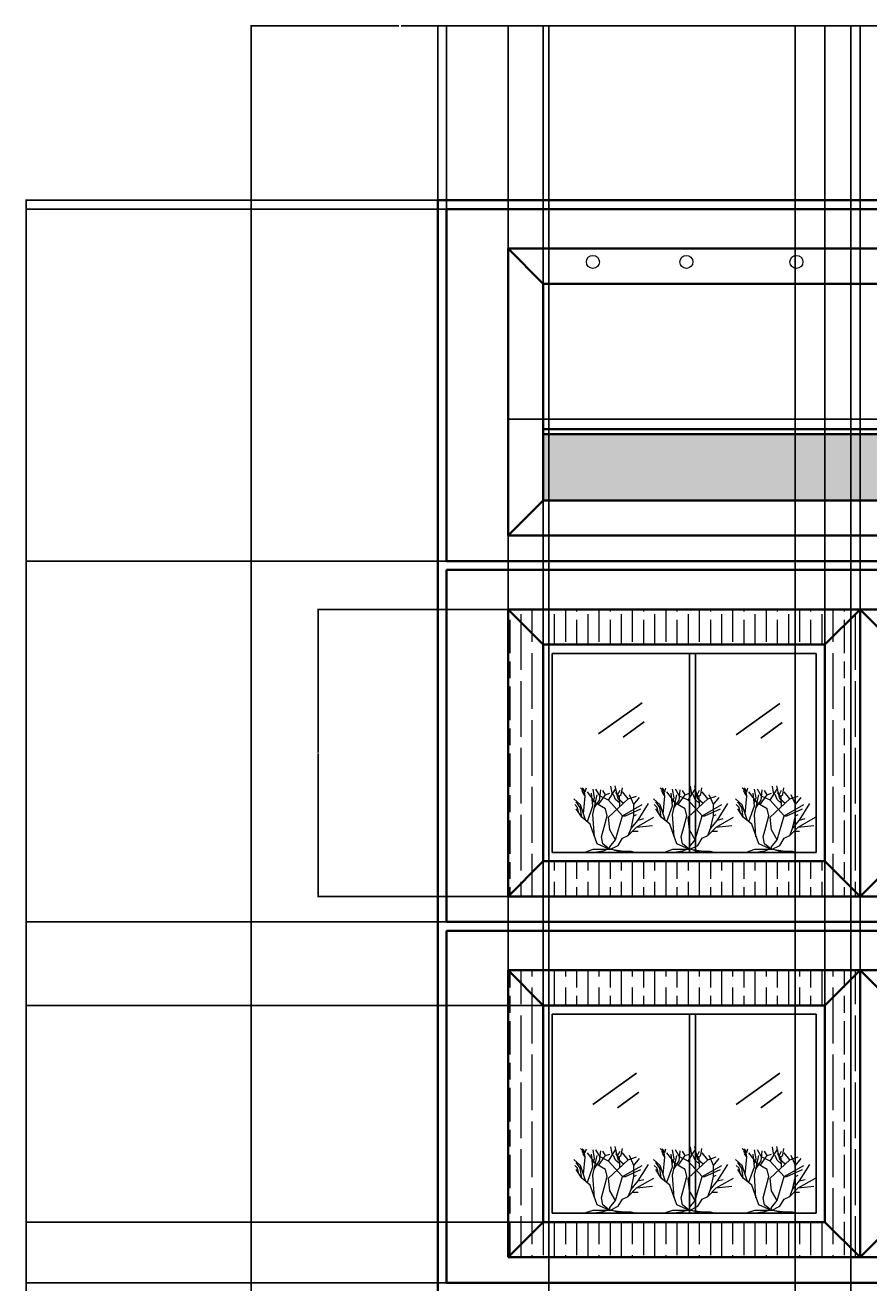
# Model space of a CAD drawing. Units: inches. Extents: x -97 to 1206, y -378 to 680.
# Tile 4 of 6: x -97 to 191, y 251 to 680. Entities that reach past the tile are written whole.
import ezdxf

# ---------------------------------------------------------------- set-up
doc = ezdxf.new("R2010")
doc.units = ezdxf.units.IN
doc.header["$MEASUREMENT"] = 0
for name, color, linetype, lineweight in [('A-ANNO-DIMS', 2, 'Continuous', 18), ('A-ELEV', 7, 'Continuous', 35), ('A-ELEV-PATT', 252, 'Continuous', 13), ('A-GLAZ', 4, 'Continuous', 25), ('E-LITE', 2, 'Continuous', 18), ('L-PLNT', 82, 'Continuous', 13)]:
    doc.layers.add(name, color=color, linetype=linetype, lineweight=lineweight)
doc.styles.get("Standard").update_dxf_attribs({"font": 'arial.ttf'})
doc.dimstyles.get("Standard").update_dxf_attribs({"dimtxt": 0.18, "dimasz": 0.18, "dimexe": 0.18, "dimexo": 0.0625, "dimgap": 0.09, "dimtad": 0, "dimtih": 1, "dimtoh": 1, "dimdec": 4, "dimzin": 0, "dimdsep": 46, "dimtxsty": 'Standard', "dimcen": 0.09, "dimadec": 0, "dimazin": 0, "dimtfac": 1, "dimtdec": 4, "dimtofl": 0, "dimtmove": 0, "dimatfit": 3, "dimfxl": 1, "dimtolj": 1, "dimtzin": 0, "dimarcsym": 0})

# ---------------------------------------------------------------- blocks, each defined once
blk = doc.blocks.new('*U2')
for p, q in [((-12.471, 19.775), (-12.898, 22.044)), ((-11.433, 18.289), (-10.457, 22.749)), ((-8.16, 17.76), (-10.56, 21.6)), ((-9.48, 19.775), (-8.992, 22.592)), ((-5.28, 19.2), (-3.84, 21.6)), ((-3.377, 18.602), (-2.888, 21.575)), ((-0.508, 21.888), (-0.081, 20.558)), ((0.041, 20.714), (1.384, 22.044)), ((0.102, 21.34), (0.835, 21.888)), ((-16.8, 16.32), (-18.72, 18.72)), ((-14.88, 18.24), (-17.76, 19.2)), ((-16.8, 16.32), (-15.36, 19.68)), ((-14.88, 18.24), (-12.96, 20.64)), ((-8.16, 12), (-14.88, 18.24)), ((-13.325, 16.724), (-11.433, 18.289)), ((-12.96, 12.48), (-8.16, 17.76)), ((-11.677, 19.071), (-12.471, 19.775)), ((-11.28, 19.619), (-12.104, 21.184)), ((-12.043, 15.628), (-11.921, 18.836)), ((-11.982, 16.802), (-10.579, 18.054)), ((-11.921, 18.836), (-10.64, 20.401)), ((-10.579, 18.054), (-9.846, 19.697)), ((-7.2, 19.68), (-8.64, 20.16)), ((-8.16, 17.76), (-5.28, 19.2)), ((-7.2, 19.68), (-6.24, 21.12)), ((-4.8, 16.32), (-7.2, 19.68)), ((-5.086, 17.741), (-5.513, 21.34)), ((-3.377, 15.315), (-5.086, 17.819)), ((-2.88, 12.96), (-4.32, 19.68)), ((-3.84, 16.8), (-0.96, 20.64)), ((-2.766, 16.802), (-3.377, 18.602)), ((-2.88, 15.84), (-2.4, 20.16)), ((-0.203, 19.149), (0.102, 21.34)), ((0.346, 13.203), (-0.203, 19.149)), ((-0.142, 19.384), (0.59, 20.401)), ((-0.02, 20.01), (0.896, 21.105)), ((1.323, 16.254), (3.642, 18.289)), ((1.44, 15.36), (2.88, 17.28)), ((-18.24, 11.04), (-21.755, 16.655)), ((-12.96, 12.48), (-19.68, 16.32)), ((-13.92, 12.48), (-19.2, 14.88)), ((-16.8, 12.48), (-17.76, 12.96)), ((-16.8, 12.48), (-16.8, 16.32)), ((-7.68, 12.48), (-7.2, 14.88)), ((-7.2, 14.88), (-3.84, 16.8)), ((-3.36, 5.28), (-2.88, 12.96)), ((-0.96, 10.56), (-2.88, 15.84)), ((-0.48, 10.8), (0.346, 13.203)), ((0.346, 13.203), (1.323, 16.254)), ((0.96, 12), (1.44, 15.36)), ((0.96, 12), (2.88, 14.88)), ((1.92, 13.44), (2.4, 15.36)), ((2.4, 15.36), (3.36, 16.32)), ((-17.76, 8.64), (-23.663, 11.961)), ((-17.76, 8.64), (-23.128, 9.222)), ((-18.24, 11.04), (-20.16, 11.52)), ((-15.84, 8.16), (-18.24, 11.04)), ((-14.88, 5.76), (-17.76, 8.64)), ((-15.84, 8.16), (-16.8, 12.48)), ((-12.96, 12.48), (-13.92, 12.48)), ((-10.56, 4.32), (-12.96, 12.48)), ((-8.64, 7.68), (-8.16, 12)), ((-6.72, 8.64), (-7.68, 12.48)), ((-5.76, 5.28), (-6.72, 8.64)), ((-4.32, 2.88), (-1.92, 9.6)), ((-1.92, 9.6), (0.96, 12)), ((-16.32, 7.2), (-18.24, 7.2)), ((-14.88, 5.76), (-15.84, 8.16)), ((-12.96, 4.8), (-14.88, 5.76)), ((-11.52, 2.4), (-12.96, 4.8)), ((-10.56, 4.32), (-8.64, 7.68)), ((-8.64, 1.92), (-10.56, 4.32)), ((-6.24, 2.88), (-5.76, 5.28)), ((-15.84, 0.48), (-17.76, 0)), ((-13.44, 0.48), (-15.84, 0.48)), ((-9.6, 0.96), (-13.44, 0.48)), ((-9.6, 0.96), (-12.96, 0)), ((-8.64, 0.96), (-11.52, 2.4)), ((-9.6, 0.96), (-7.68, 0.96)), ((-8.64, 0.96), (-4.32, 2.88)), ((-8.64, 0.96), (-6.24, 2.88)), ((-8.64, 0.96), (-8.64, 1.92)), ((-8.64, 0.96), (-2.88, 0.96)), ((-7.68, 0.96), (-6.24, 0.48)), ((-6.24, 0.48), (-3.36, 0)), ((-2.88, 0.96), (0, 0))]:
    blk.add_line(p, q)
blk = doc.blocks.new('FACADE-SURROUND')
for p, q in [((432, 97.83), (0, 97.83)), ((0, 97.83), (0, 0)), ((12, 85.83), (0, 97.83)), ((300, 85.83), (312, 97.83)), ((312, 0), (312, 97.83)), ((312, 0), (312, 97.83)), ((312, 97.83), (324, 85.83)), ((432, 97.83), (420, 85.83)), ((432, 0), (432, 97.83)), ((12, 85.83), (12, 12)), ((108, 85.83), (12, 85.83)), ((300, 85.83), (126, 85.83)), ((126, 85.83), (126, 12)), ((300, 12), (300, 85.83)), ((324, 12), (324, 85.83)), ((420, 85.83), (324, 85.83)), ((420, 12), (420, 85.83)), ((12, 12), (0, 0)), ((12, 12), (108, 12)), ((126, 12), (300, 12)), ((300, 12), (312, 0)), ((312, 0), (324, 12)), ((324, 12), (420, 12)), ((432, 0), (420, 12)), ((0, 0), (432, 0))]:
    blk.add_line(p, q)
blk = doc.blocks.new('WIN-1500')
for p, q in [((90, 67.83), (0, 67.83)), ((0, 67.83), (0, 0)), ((90, 67.83), (90, 0)), ((0, 0), (90, 0))]:
    blk.add_line(p, q)
blk = doc.blocks.new('*D9')
at = {"layer": 'A-ANNO-DIMS', "color": 0, "lineweight": -2, "transparency": 16777216}
for p, q in [((67.93, 480.46), (67.93, 545.38)), ((68.11, 545.2), (282.03, 545.2)), ((499.75, 545.2), (285.83, 545.2)), ((499.93, 480.46), (499.93, 545.38))]:
    blk.add_line(p, q, dxfattribs=at)
at = {"layer": 'A-ANNO-DIMS', "color": 0, "transparency": 16777216}
for points in [[(68.11, 545.23), (68.11, 545.17), (67.93, 545.2)], [(499.75, 545.23), (499.75, 545.17), (499.93, 545.2)]]:
    blk.add_solid(points, dxfattribs=at)
at = {"layer": 'Defpoints', "color": 0, "transparency": 16777216}
for p in [(67.93, 545.2), (67.93, 480.4), (499.93, 480.4)]:
    blk.add_point(p, dxfattribs=at)
at = {"layer": 'A-ANNO-DIMS', "color": 0, "transparency": 16777216, "insert": (283.93, 545.2), "char_height": 0.18, "attachment_point": 5}
blk.add_mtext('\\A1;FACADE SURROUND 432 TYP.', dxfattribs=at)
blk = doc.blocks.new('*D10')
at = {"layer": 'A-ANNO-DIMS', "color": 0, "lineweight": -2, "transparency": 16777216}
for p, q in [((67.86, 480.4), (2.95, 480.4)), ((3.13, 480.22), (3.13, 431.66)), ((3.13, 382.75), (3.13, 431.3)), ((67.86, 382.57), (2.95, 382.57))]:
    blk.add_line(p, q, dxfattribs=at)
at = {"layer": 'A-ANNO-DIMS', "color": 0, "transparency": 16777216}
for points in [[(3.1, 480.22), (3.16, 480.22), (3.13, 480.4)], [(3.1, 382.75), (3.16, 382.75), (3.13, 382.57)]]:
    blk.add_solid(points, dxfattribs=at)
at = {"layer": 'Defpoints', "color": 0, "transparency": 16777216}
for p in [(67.93, 480.4), (3.13, 382.57), (67.93, 382.57)]:
    blk.add_point(p, dxfattribs=at)
at = {"layer": 'A-ANNO-DIMS', "color": 0, "transparency": 16777216, "insert": (3.13, 431.48), "char_height": 0.18, "attachment_point": 5}
blk.add_mtext('\\A1;98 TYP.', dxfattribs=at)
blk = doc.blocks.new('*D12')
at = {"layer": 'A-ANNO-DIMS', "color": 0, "lineweight": -2, "transparency": 16777216}
for p, q in [((43.86, 619.86), (-96.59, 619.86)), ((-96.41, 619.68), (-96.41, 252.54)), ((-96.41, -114.96), (-96.41, 252.17)), ((-36.97, -115.14), (-96.59, -115.14))]:
    blk.add_line(p, q, dxfattribs=at)
at = {"layer": 'A-ANNO-DIMS', "color": 0, "transparency": 16777216}
for points in [[(-96.44, 619.68), (-96.38, 619.68), (-96.41, 619.86)], [(-96.44, -114.96), (-96.38, -114.96), (-96.41, -115.14)]]:
    blk.add_solid(points, dxfattribs=at)
at = {"layer": 'Defpoints', "color": 0, "transparency": 16777216}
for p in [(43.93, 619.86), (-96.41, -115.14), (-36.91, -115.14)]:
    blk.add_point(p, dxfattribs=at)
at = {"layer": 'A-ANNO-DIMS', "color": 0, "transparency": 16777216, "insert": (-96.41, 252.36), "char_height": 0.18, "attachment_point": 5}
blk.add_mtext('\\A1;735', dxfattribs=at)
blk = doc.blocks.new('*D16')
at = {"layer": 'A-ANNO-DIMS', "color": 0, "lineweight": -2, "transparency": 16777216}
for p, q in [((46.86, 373.86), (-96.59, 373.86)), ((-96.41, 373.68), (-96.41, 312.54)), ((-96.41, 251.04), (-96.41, 312.17)), ((46.86, 250.86), (-96.59, 250.86))]:
    blk.add_line(p, q, dxfattribs=at)
at = {"layer": 'A-ANNO-DIMS', "color": 0, "transparency": 16777216}
for points in [[(-96.44, 373.68), (-96.38, 373.68), (-96.41, 373.86)], [(-96.44, 251.04), (-96.38, 251.04), (-96.41, 250.86)]]:
    blk.add_solid(points, dxfattribs=at)
at = {"layer": 'Defpoints', "color": 0, "transparency": 16777216}
for p in [(-96.41, 373.86), (46.93, 373.86), (46.93, 250.86)]:
    blk.add_point(p, dxfattribs=at)
at = {"layer": 'A-ANNO-DIMS', "color": 0, "transparency": 16777216, "insert": (-96.41, 312.36), "char_height": 0.18, "attachment_point": 5}
blk.add_mtext('\\A1;123', dxfattribs=at)
blk = doc.blocks.new('*D17')
at = {"layer": 'A-ANNO-DIMS', "color": 0, "lineweight": -2, "transparency": 16777216}
for p, q in [((46.86, 496.86), (-96.59, 496.86)), ((-96.41, 496.68), (-96.41, 435.54)), ((-96.41, 374.04), (-96.41, 435.17)), ((46.86, 373.86), (-96.59, 373.86))]:
    blk.add_line(p, q, dxfattribs=at)
at = {"layer": 'A-ANNO-DIMS', "color": 0, "transparency": 16777216}
for points in [[(-96.44, 496.68), (-96.38, 496.68), (-96.41, 496.86)], [(-96.44, 374.04), (-96.38, 374.04), (-96.41, 373.86)]]:
    blk.add_solid(points, dxfattribs=at)
at = {"layer": 'Defpoints', "color": 0, "transparency": 16777216}
for p in [(-96.41, 496.86), (46.93, 496.86), (46.93, 373.86)]:
    blk.add_point(p, dxfattribs=at)
at = {"layer": 'A-ANNO-DIMS', "color": 0, "transparency": 16777216, "insert": (-96.41, 435.36), "char_height": 0.18, "attachment_point": 5}
blk.add_mtext('\\A1;123', dxfattribs=at)
blk = doc.blocks.new('*D18')
at = {"layer": 'A-ANNO-DIMS', "color": 0, "lineweight": -2, "transparency": 16777216}
for p, q in [((46.86, 616.86), (-96.59, 616.86)), ((-96.41, 616.68), (-96.41, 557.04)), ((-96.41, 497.04), (-96.41, 556.67)), ((46.86, 496.86), (-96.59, 496.86))]:
    blk.add_line(p, q, dxfattribs=at)
at = {"layer": 'A-ANNO-DIMS', "color": 0, "transparency": 16777216}
for points in [[(-96.44, 616.68), (-96.38, 616.68), (-96.41, 616.86)], [(-96.44, 497.04), (-96.38, 497.04), (-96.41, 496.86)]]:
    blk.add_solid(points, dxfattribs=at)
at = {"layer": 'Defpoints', "color": 0, "transparency": 16777216}
for p in [(-96.41, 616.86), (46.93, 616.86), (46.93, 496.86)]:
    blk.add_point(p, dxfattribs=at)
at = {"layer": 'A-ANNO-DIMS', "color": 0, "transparency": 16777216, "insert": (-96.41, 556.86), "char_height": 0.18, "attachment_point": 5}
blk.add_mtext('\\A1;120', dxfattribs=at)
blk = doc.blocks.new('*D31')
at = {"layer": 'A-ANNO-DIMS', "color": 0, "lineweight": -2, "transparency": 16777216}
for p, q in [((46.93, 616.92), (46.93, 679.54)), ((47.11, 679.36), (57.22, 679.36)), ((67.75, 679.36), (57.63, 679.36)), ((67.93, 603.46), (67.93, 679.54))]:
    blk.add_line(p, q, dxfattribs=at)
at = {"layer": 'A-ANNO-DIMS', "color": 0, "transparency": 16777216}
for points in [[(47.11, 679.39), (47.11, 679.33), (46.93, 679.36)], [(67.75, 679.39), (67.75, 679.33), (67.93, 679.36)]]:
    blk.add_solid(points, dxfattribs=at)
at = {"layer": 'Defpoints', "color": 0, "transparency": 16777216}
for p in [(67.93, 679.36), (46.93, 616.86), (67.93, 603.4)]:
    blk.add_point(p, dxfattribs=at)
at = {"layer": 'A-ANNO-DIMS', "color": 0, "transparency": 16777216, "insert": (57.43, 679.36), "char_height": 0.18, "attachment_point": 5}
blk.add_mtext('\\A1;21', dxfattribs=at)
blk = doc.blocks.new('*D32')
at = {"layer": 'A-ANNO-DIMS', "color": 0, "lineweight": -2, "transparency": 16777216}
for p, q in [((67.93, 603.46), (67.93, 679.54)), ((68.11, 679.36), (229.64, 679.36)), ((391.75, 679.36), (230.21, 679.36)), ((391.93, 603.46), (391.93, 679.54))]:
    blk.add_line(p, q, dxfattribs=at)
at = {"layer": 'A-ANNO-DIMS', "color": 0, "transparency": 16777216}
for points in [[(68.11, 679.39), (68.11, 679.33), (67.93, 679.36)], [(391.75, 679.39), (391.75, 679.33), (391.93, 679.36)]]:
    blk.add_solid(points, dxfattribs=at)
at = {"layer": 'Defpoints', "color": 0, "transparency": 16777216}
for p in [(391.93, 679.36), (67.93, 603.4), (391.93, 603.4)]:
    blk.add_point(p, dxfattribs=at)
at = {"layer": 'A-ANNO-DIMS', "color": 0, "transparency": 16777216, "insert": (229.93, 679.36), "char_height": 0.18, "attachment_point": 5}
blk.add_mtext('\\A1;324', dxfattribs=at)
blk = doc.blocks.new('*D36')
at = {"layer": 'A-ANNO-DIMS', "color": 0, "lineweight": -2, "transparency": 16777216}
for p, q in [((-19.68, -48.26), (-19.68, 679.54)), ((-19.5, 679.36), (30.69, 679.36)), ((81.65, 679.36), (31.46, 679.36)), ((81.83, -48.26), (81.83, 679.54))]:
    blk.add_line(p, q, dxfattribs=at)
at = {"layer": 'A-ANNO-DIMS', "color": 0, "transparency": 16777216}
for points in [[(-19.5, 679.39), (-19.5, 679.33), (-19.68, 679.36)], [(81.65, 679.39), (81.65, 679.33), (81.83, 679.36)]]:
    blk.add_solid(points, dxfattribs=at)
at = {"layer": 'Defpoints', "color": 0, "transparency": 16777216}
for p in [(81.83, 679.36), (-19.68, -48.33), (81.83, -48.33)]:
    blk.add_point(p, dxfattribs=at)
at = {"layer": 'A-ANNO-DIMS', "color": 0, "transparency": 16777216, "insert": (31.08, 679.36), "char_height": 0.18, "attachment_point": 5}
blk.add_mtext('\\A1;101.5', dxfattribs=at)
blk = doc.blocks.new('*D45')
at = {"layer": 'A-ANNO-DIMS', "color": 0, "lineweight": -2, "transparency": 16777216}
for p, q in [((43.93, -24.66), (43.93, 679.54)), ((44.11, 679.36), (104.5, 679.36)), ((165.65, 679.36), (105.27, 679.36)), ((165.83, -24.66), (165.83, 679.54))]:
    blk.add_line(p, q, dxfattribs=at)
at = {"layer": 'A-ANNO-DIMS', "color": 0, "transparency": 16777216}
for points in [[(44.11, 679.39), (44.11, 679.33), (43.93, 679.36)], [(165.65, 679.39), (165.65, 679.33), (165.83, 679.36)]]:
    blk.add_solid(points, dxfattribs=at)
at = {"layer": 'Defpoints', "color": 0, "transparency": 16777216}
for p in [(165.83, 679.36), (43.93, -24.73), (165.83, -24.73)]:
    blk.add_point(p, dxfattribs=at)
at = {"layer": 'A-ANNO-DIMS', "color": 0, "transparency": 16777216, "insert": (104.88, 679.36), "char_height": 0.18, "attachment_point": 5}
blk.add_mtext('\\A1;121.9', dxfattribs=at)
blk = doc.blocks.new('*D46')
at = {"layer": 'A-ANNO-DIMS', "color": 0, "lineweight": -2, "transparency": 16777216}
for p, q in [((165.83, -24.66), (165.83, 679.54)), ((166.01, 679.36), (174.88, 679.36)), ((184.65, 679.36), (175.79, 679.36)), ((184.83, -24.66), (184.83, 679.54))]:
    blk.add_line(p, q, dxfattribs=at)
at = {"layer": 'A-ANNO-DIMS', "color": 0, "transparency": 16777216}
for points in [[(166.01, 679.39), (166.01, 679.33), (165.83, 679.36)], [(184.65, 679.39), (184.65, 679.33), (184.83, 679.36)]]:
    blk.add_solid(points, dxfattribs=at)
at = {"layer": 'Defpoints', "color": 0, "transparency": 16777216}
for p in [(184.83, 679.36), (165.83, -24.73), (184.83, -24.73)]:
    blk.add_point(p, dxfattribs=at)
at = {"layer": 'A-ANNO-DIMS', "color": 0, "transparency": 16777216, "insert": (175.33, 679.36), "char_height": 0.18, "attachment_point": 5}
blk.add_mtext('\\A1;18.994', dxfattribs=at)
blk = doc.blocks.new('*D47')
at = {"layer": 'A-ANNO-DIMS', "color": 0, "lineweight": -2, "transparency": 16777216}
for p, q in [((184.83, -24.66), (184.83, 679.54)), ((185.01, 679.36), (255.01, 679.36)), ((325.75, 679.36), (255.75, 679.36)), ((325.93, -24.66), (325.93, 679.54))]:
    blk.add_line(p, q, dxfattribs=at)
at = {"layer": 'A-ANNO-DIMS', "color": 0, "transparency": 16777216}
for points in [[(185.01, 679.39), (185.01, 679.33), (184.83, 679.36)], [(325.75, 679.39), (325.75, 679.33), (325.93, 679.36)]]:
    blk.add_solid(points, dxfattribs=at)
at = {"layer": 'Defpoints', "color": 0, "transparency": 16777216}
for p in [(325.93, 679.36), (184.83, -24.73), (325.93, -24.73)]:
    blk.add_point(p, dxfattribs=at)
at = {"layer": 'A-ANNO-DIMS', "color": 0, "transparency": 16777216, "insert": (255.38, 679.36), "char_height": 0.18, "attachment_point": 5}
blk.add_mtext('\\A1;141.1', dxfattribs=at)
blk = doc.blocks.new('*D51')
at = {"layer": 'A-ANNO-DIMS', "color": 0, "lineweight": -2, "transparency": 16777216}
for p, q in [((67.93, 357.46), (67.93, 679.54)), ((68.11, 679.36), (73.54, 679.36)), ((79.75, 679.36), (74.31, 679.36)), ((79.93, 345.46), (79.93, 679.54))]:
    blk.add_line(p, q, dxfattribs=at)
at = {"layer": 'A-ANNO-DIMS', "color": 0, "transparency": 16777216}
for points in [[(68.11, 679.39), (68.11, 679.33), (67.93, 679.36)], [(79.75, 679.39), (79.75, 679.33), (79.93, 679.36)]]:
    blk.add_solid(points, dxfattribs=at)
at = {"layer": 'Defpoints', "color": 0, "transparency": 16777216}
for p in [(79.93, 679.36), (67.93, 357.4), (79.93, 345.4)]:
    blk.add_point(p, dxfattribs=at)
at = {"layer": 'A-ANNO-DIMS', "color": 0, "transparency": 16777216, "insert": (73.93, 679.36), "char_height": 0.18, "attachment_point": 5}
blk.add_mtext('\\A1;12.00', dxfattribs=at)
blk = doc.blocks.new('*D52')
at = {"layer": 'A-ANNO-DIMS', "color": 0, "lineweight": -2, "transparency": 16777216}
for p, q in [((79.93, 345.46), (79.93, 679.54)), ((80.11, 679.36), (127.53, 679.36)), ((175.75, 679.36), (128.32, 679.36)), ((175.93, 345.46), (175.93, 679.54))]:
    blk.add_line(p, q, dxfattribs=at)
at = {"layer": 'A-ANNO-DIMS', "color": 0, "transparency": 16777216}
for points in [[(80.11, 679.39), (80.11, 679.33), (79.93, 679.36)], [(175.75, 679.39), (175.75, 679.33), (175.93, 679.36)]]:
    blk.add_solid(points, dxfattribs=at)
at = {"layer": 'Defpoints', "color": 0, "transparency": 16777216}
for p in [(175.93, 679.36), (79.93, 345.4), (175.93, 345.4)]:
    blk.add_point(p, dxfattribs=at)
at = {"layer": 'A-ANNO-DIMS', "color": 0, "transparency": 16777216, "insert": (127.93, 679.36), "char_height": 0.18, "attachment_point": 5}
blk.add_mtext('\\A1;96.00', dxfattribs=at)
blk = doc.blocks.new('*D53')
at = {"layer": 'A-ANNO-DIMS', "color": 0, "lineweight": -2, "transparency": 16777216}
for p, q in [((175.86, 345.4), (-96.59, 345.4)), ((-96.41, 345.22), (-96.41, 308.66)), ((-96.41, 271.75), (-96.41, 308.3)), ((175.86, 271.57), (-96.59, 271.57))]:
    blk.add_line(p, q, dxfattribs=at)
at = {"layer": 'A-ANNO-DIMS', "color": 0, "transparency": 16777216}
for points in [[(-96.44, 345.22), (-96.38, 345.22), (-96.41, 345.4)], [(-96.44, 271.75), (-96.38, 271.75), (-96.41, 271.57)]]:
    blk.add_solid(points, dxfattribs=at)
at = {"layer": 'Defpoints', "color": 0, "transparency": 16777216}
for p in [(-96.41, 345.4), (175.93, 345.4), (175.93, 271.57)]:
    blk.add_point(p, dxfattribs=at)
at = {"layer": 'A-ANNO-DIMS', "color": 0, "transparency": 16777216, "insert": (-96.41, 308.48), "char_height": 0.18, "attachment_point": 5}
blk.add_mtext('\\A1;73.83', dxfattribs=at)
blk = doc.blocks.new('*D54')
at = {"layer": 'A-ANNO-DIMS', "color": 0, "lineweight": -2, "transparency": 16777216}
for p, q in [((67.93, 259.63), (67.93, 679.54)), ((68.11, 679.36), (127.47, 679.36)), ((187.75, 679.36), (128.38, 679.36)), ((187.93, 259.63), (187.93, 679.54))]:
    blk.add_line(p, q, dxfattribs=at)
at = {"layer": 'A-ANNO-DIMS', "color": 0, "transparency": 16777216}
for points in [[(68.11, 679.39), (68.11, 679.33), (67.93, 679.36)], [(187.75, 679.39), (187.75, 679.33), (187.93, 679.36)]]:
    blk.add_solid(points, dxfattribs=at)
at = {"layer": 'Defpoints', "color": 0, "transparency": 16777216}
for p in [(187.93, 679.36), (67.93, 259.57), (187.93, 259.57)]:
    blk.add_point(p, dxfattribs=at)
at = {"layer": 'A-ANNO-DIMS', "color": 0, "transparency": 16777216, "insert": (127.93, 679.36), "char_height": 0.18, "attachment_point": 5}
blk.add_mtext('\\A1;120.00', dxfattribs=at)

msp = doc.modelspace()

# ---------------------------------------------------------------- hatches: boundary and pattern name
at = {"layer": 'A-ELEV-PATT'}
h = msp.add_hatch(dxfattribs=at)
h.set_pattern_fill('GOST_GLASS', color=256)
h.set_pattern_definition([(45, (-208.809, -191.922), (8.48528, 0), [5, -7]), (45, (-206.6876, -191.922), (8.48528, 0), [2, -10]), (45, (-208.809, -189.8007), (8.48528, 0), [2, -10])])
h.paths.add_polyline_path([(225.9926, 155.8067), (224.5809, 157.6166), (220.3456, 160.3315), (219.9926, 160.3315), (218.5808, 160.7839), (218.5808, 162.3676), (217.6985, 163.4988), (216.4631, 162.8201), (212.4043, 157.8428), (211.522, 157.8428), (209.4043, 162.3676), (206.4043, 161.0102), (205.169, 161.9151), (198.6395, 161.6889), (197.5807, 163.4988), (200.2278, 166.4399), (201.816, 167.3448), (205.3454, 167.5711), (208.0494, 171.1321), (193.9261, 171.1321), (193.9261, 148.5671), (225.6397, 148.5671), (226.3455, 153.3181)])
h.paths.add_polyline_path([(228.9926, 165.5349), (229.6985, 165.0825), (230.2279, 163.2726), (231.4632, 163.9513), (231.8162, 163.4988), (232.1691, 162.3676), (233.4044, 164.4038), (234.6397, 164.4038), (235.1691, 163.4988), (234.6397, 162.5939), (236.0515, 163.0463), (236.5809, 162.3676), (237.8162, 163.2726), (239.0515, 162.8201), (241.5221, 160.3315), (242.5809, 159.879), (243.4633, 158.974), (250.8751, 159.6527), (252.2869, 158.2953), (253.3457, 158.7478), (250.5222, 162.3676), (250.3457, 163.725), (251.2281, 165.0825), (249.6398, 169.381), (248.7575, 169.381), (248.2696, 171.1321), (208.0494, 171.1321), (205.3454, 167.5711), (201.816, 167.3448), (200.2278, 166.4399), (197.5807, 163.4988), (198.6395, 161.6889), (205.169, 161.9151), (206.4043, 161.0102), (209.4043, 162.3676), (211.522, 157.8428), (212.4043, 157.8428), (216.4631, 162.8201), (217.6985, 163.4988), (218.5808, 162.3676), (218.5808, 160.7839), (219.9926, 160.3315), (221.9338, 160.3315), (222.6396, 161.9151), (224.9338, 163.0463), (227.228, 163.2726), (228.2868, 164.1775), (228.4632, 164.4038)])
h.paths.add_polyline_path([(236.7574, 156.033), (239.7468, 162.1197), (239.0515, 162.8201), (237.8162, 163.2726), (236.5809, 162.3676), (236.0515, 163.0463), (234.6397, 162.5939), (235.1691, 163.4988), (234.6397, 164.4038), (233.4044, 164.4038), (232.1691, 162.3676), (231.8162, 163.4988), (231.4632, 163.9513), (230.2279, 163.2726), (229.6985, 165.0825), (228.9926, 165.5349), (228.4632, 164.4038), (228.2868, 164.1775), (227.228, 163.2726), (224.9338, 163.0463), (222.6396, 161.9151), (221.9338, 160.3315), (220.3456, 160.3315), (224.5809, 157.6166), (225.9926, 155.8067), (226.3455, 153.3181), (225.6397, 148.5671), (228.9926, 148.5671), (228.8162, 150.1507), (229.3456, 152.8656)])
h.paths.add_polyline_path([(367.9261, 171.1321), (248.2696, 171.1321), (248.7575, 169.381), (249.6398, 169.381), (251.2281, 165.0825), (250.3457, 163.725), (250.5222, 162.3676), (253.3457, 158.7478), (252.2869, 158.2953), (250.8751, 159.6527), (243.4633, 158.974), (242.5809, 159.879), (241.5221, 160.3315), (239.7468, 162.1197), (236.7574, 156.033), (229.3456, 152.8656), (228.8162, 150.1507), (228.9926, 148.5671), (367.9261, 148.5671)])
h.paths.add_polyline_path([(367.9261, 48.1321), (237.8147, 48.1321), (238.3026, 46.381), (239.1849, 46.381), (240.7732, 42.0825), (239.8908, 40.725), (240.0673, 39.3676), (242.8908, 35.7478), (241.832, 35.2953), (240.4202, 36.6527), (233.0084, 35.974), (232.126, 36.879), (231.0672, 37.3315), (229.2919, 39.1197), (226.3025, 33.033), (218.8907, 29.8656), (218.3613, 27.1507), (218.5377, 25.5671), (367.9261, 25.5671)])
h.paths.add_polyline_path([(226.3025, 33.033), (229.2919, 39.1197), (228.5966, 39.8201), (227.3613, 40.2726), (226.126, 39.3676), (225.5966, 40.0463), (224.1848, 39.5939), (224.7142, 40.4988), (224.1848, 41.4038), (222.9495, 41.4038), (221.7142, 39.3676), (221.3613, 40.4988), (221.0083, 40.9513), (219.7731, 40.2726), (219.2436, 42.0825), (218.5377, 42.5349), (218.0083, 41.4038), (217.8319, 41.1775), (216.7731, 40.2726), (214.4789, 40.0463), (212.1847, 38.9151), (211.4789, 37.3315), (209.8907, 37.3315), (214.126, 34.6166), (215.5377, 32.8067), (215.8907, 30.3181), (215.1848, 25.5671), (218.5377, 25.5671), (218.3613, 27.1507), (218.8907, 29.8656)])
h.paths.add_polyline_path([(239.1849, 46.381), (238.3026, 46.381), (237.8147, 48.1321), (197.5945, 48.1321), (194.8905, 44.5711), (193.9261, 44.5093), (193.9261, 38.8878), (194.7141, 38.9151), (195.9494, 38.0102), (198.9494, 39.3676), (201.0671, 34.8428), (201.9494, 34.8428), (206.0083, 39.8201), (207.2436, 40.4988), (208.1259, 39.3676), (208.1259, 37.7839), (209.5377, 37.3315), (211.4789, 37.3315), (212.1847, 38.9151), (214.4789, 40.0463), (216.7731, 40.2726), (217.8319, 41.1775), (218.0083, 41.4038), (218.5377, 42.5349), (219.2436, 42.0825), (219.7731, 40.2726), (221.0083, 40.9513), (221.3613, 40.4988), (221.7142, 39.3676), (222.9495, 41.4038), (224.1848, 41.4038), (224.7142, 40.4988), (224.1848, 39.5939), (225.5966, 40.0463), (226.126, 39.3676), (227.3613, 40.2726), (228.5966, 39.8201), (231.0672, 37.3315), (232.126, 36.879), (233.0084, 35.974), (240.4202, 36.6527), (241.832, 35.2953), (242.8908, 35.7478), (240.0673, 39.3676), (239.8908, 40.725), (240.7732, 42.0825)])
h.paths.add_polyline_path([(215.5377, 32.8067), (214.126, 34.6166), (209.8907, 37.3315), (209.5377, 37.3315), (208.1259, 37.7839), (208.1259, 39.3676), (207.2436, 40.4988), (206.0083, 39.8201), (201.9494, 34.8428), (201.0671, 34.8428), (198.9494, 39.3676), (195.9494, 38.0102), (194.7141, 38.9151), (193.9261, 38.8878), (193.9261, 25.5671), (215.1848, 25.5671), (215.8907, 30.3181)])
h.paths.add_polyline_path([(336.7518, 280.6166), (332.5165, 283.3315), (332.1636, 283.3315), (330.7518, 283.7839), (330.7518, 285.3676), (329.8694, 286.4988), (328.6341, 285.8201), (324.5753, 280.8428), (323.6929, 280.8428), (321.5753, 285.3676), (318.5752, 284.0102), (317.3399, 284.9151), (310.8105, 284.6889), (309.7516, 286.4988), (312.3987, 289.4399), (313.987, 290.3448), (317.5164, 290.5711), (320.2203, 294.1321), (199.9261, 294.1321), (199.9261, 271.5671), (337.8106, 271.5671), (338.5165, 276.3181), (338.1636, 278.8067)])
h.paths.add_polyline_path([(321.5753, 408.3676), (318.5752, 407.0102), (317.3399, 407.9151), (310.8105, 407.6889), (309.7516, 409.4988), (312.3987, 412.4399), (313.987, 413.3448), (317.5164, 413.5711), (320.2203, 417.1321), (199.9261, 417.1321), (199.9261, 394.5671), (337.8106, 394.5671), (338.5165, 399.3181), (338.1636, 401.8067), (336.7518, 403.6166), (332.5165, 406.3315), (332.1636, 406.3315), (330.7518, 406.7839), (330.7518, 408.3676), (329.8694, 409.4988), (328.6341, 408.8201), (324.5753, 403.8428), (323.6929, 403.8428)])
h.paths.add_polyline_path([(373.9261, 540.1321), (79.9261, 540.1321), (79.9261, 517.5671), (373.9261, 517.5671)])
h.paths.add_polyline_path([(373.9261, 417.1321), (360.4406, 417.1321), (360.9284, 415.381), (361.8108, 415.381), (363.399, 411.0825), (362.5167, 409.725), (362.6931, 408.3676), (365.5167, 404.7478), (364.4578, 404.2953), (363.0461, 405.6527), (355.6343, 404.974), (354.7519, 405.879), (353.6931, 406.3315), (351.9178, 408.1197), (348.9284, 402.033), (341.5166, 398.8656), (340.9871, 396.1507), (341.1636, 394.5671), (373.9261, 394.5671)])
h.paths.add_polyline_path([(361.8108, 415.381), (360.9284, 415.381), (360.4406, 417.1321), (320.2203, 417.1321), (317.5164, 413.5711), (313.987, 413.3448), (312.3987, 412.4399), (309.7516, 409.4988), (310.8105, 407.6889), (317.3399, 407.9151), (318.5752, 407.0102), (321.5753, 408.3676), (323.6929, 403.8428), (324.5753, 403.8428), (328.6341, 408.8201), (329.8694, 409.4988), (330.7518, 408.3676), (330.7518, 406.7839), (332.1636, 406.3315), (334.1047, 406.3315), (334.8106, 407.9151), (337.1047, 409.0463), (339.3989, 409.2726), (340.4577, 410.1775), (340.6342, 410.4038), (341.1636, 411.5349), (341.8695, 411.0825), (342.3989, 409.2726), (343.6342, 409.9513), (343.9871, 409.4988), (344.3401, 408.3676), (345.5754, 410.4038), (346.8107, 410.4038), (347.3401, 409.4988), (346.8107, 408.5939), (348.2225, 409.0463), (348.7519, 408.3676), (349.9872, 409.2726), (351.2225, 408.8201), (353.6931, 406.3315), (354.7519, 405.879), (355.6343, 404.974), (363.0461, 405.6527), (364.4578, 404.2953), (365.5167, 404.7478), (362.6931, 408.3676), (362.5167, 409.725), (363.399, 411.0825)])
h.paths.add_polyline_path([(351.9178, 408.1197), (351.2225, 408.8201), (349.9872, 409.2726), (348.7519, 408.3676), (348.2225, 409.0463), (346.8107, 408.5939), (347.3401, 409.4988), (346.8107, 410.4038), (345.5754, 410.4038), (344.3401, 408.3676), (343.9871, 409.4988), (343.6342, 409.9513), (342.3989, 409.2726), (341.8695, 411.0825), (341.1636, 411.5349), (340.6342, 410.4038), (340.4577, 410.1775), (339.3989, 409.2726), (337.1047, 409.0463), (334.8106, 407.9151), (334.1047, 406.3315), (332.5165, 406.3315), (336.7518, 403.6166), (338.1636, 401.8067), (338.5165, 399.3181), (337.8106, 394.5671), (341.1636, 394.5671), (340.9871, 396.1507), (341.5166, 398.8656), (348.9284, 402.033)])
h.paths.add_polyline_path([(363.399, 288.0825), (361.8108, 292.381), (360.9284, 292.381), (360.4406, 294.1321), (320.2203, 294.1321), (317.5164, 290.5711), (313.987, 290.3448), (312.3987, 289.4399), (309.7516, 286.4988), (310.8105, 284.6889), (317.3399, 284.9151), (318.5752, 284.0102), (321.5753, 285.3676), (323.6929, 280.8428), (324.5753, 280.8428), (328.6341, 285.8201), (329.8694, 286.4988), (330.7518, 285.3676), (330.7518, 283.7839), (332.1636, 283.3315), (334.1047, 283.3315), (334.8106, 284.9151), (337.1047, 286.0463), (339.3989, 286.2726), (340.4577, 287.1775), (340.6342, 287.4038), (341.1636, 288.5349), (341.8695, 288.0825), (342.3989, 286.2726), (343.6342, 286.9513), (343.9871, 286.4988), (344.3401, 285.3676), (345.5754, 287.4038), (346.8107, 287.4038), (347.3401, 286.4988), (346.8107, 285.5939), (348.2225, 286.0463), (348.7519, 285.3676), (349.9872, 286.2726), (351.2225, 285.8201), (353.6931, 283.3315), (354.7519, 282.879), (355.6343, 281.974), (363.0461, 282.6527), (364.4578, 281.2953), (365.5167, 281.7478), (362.6931, 285.3676), (362.5167, 286.725)])
h.paths.add_polyline_path([(373.9261, 294.1321), (360.4406, 294.1321), (360.9284, 292.381), (361.8108, 292.381), (363.399, 288.0825), (362.5167, 286.725), (362.6931, 285.3676), (365.5167, 281.7478), (364.4578, 281.2953), (363.0461, 282.6527), (355.6343, 281.974), (354.7519, 282.879), (353.6931, 283.3315), (351.9178, 285.1197), (348.9284, 279.033), (341.5166, 275.8656), (340.9871, 273.1507), (341.1636, 271.5671), (373.9261, 271.5671)])
h.paths.add_polyline_path([(348.9284, 279.033), (351.9178, 285.1197), (351.2225, 285.8201), (349.9872, 286.2726), (348.7519, 285.3676), (348.2225, 286.0463), (346.8107, 285.5939), (347.3401, 286.4988), (346.8107, 287.4038), (345.5754, 287.4038), (344.3401, 285.3676), (343.9871, 286.4988), (343.6342, 286.9513), (342.3989, 286.2726), (341.8695, 288.0825), (341.1636, 288.5349), (340.6342, 287.4038), (340.4577, 287.1775), (339.3989, 286.2726), (337.1047, 286.0463), (334.8106, 284.9151), (334.1047, 283.3315), (332.5165, 283.3315), (336.7518, 280.6166), (338.1636, 278.8067), (338.5165, 276.3181), (337.8106, 271.5671), (341.1636, 271.5671), (340.9871, 273.1507), (341.5166, 275.8656)])
h = msp.add_hatch(dxfattribs=at)
h.set_pattern_fill('GOST_WOOD', color=256, scale=1.9)
h.set_pattern_definition([(90, (-208.809, -191.922), (11.4, -7e-16), [19, -3.8]), (90, (-205.009, -195.722), (11.4, -7e-16), [11.4, -2.85, 5.7, -2.85]), (90, (-201.209, -201.422), (11.4, -7e-16), [19, -3.8])])
h.paths.add_polyline_path([(499.9261, 111.3966), (379.9261, 111.3966), (391.9261, 99.3966), (487.9261, 99.3966)])
h.paths.add_polyline_path([(499.9261, 111.3966), (487.9261, 99.3966), (487.9261, 25.5671), (499.9261, 13.5671)])
h.paths.add_polyline_path([(487.9261, 25.5671), (391.9261, 25.5671), (379.9261, 13.5671), (499.9261, 13.5671)])
h.paths.add_polyline_path([(391.9261, 99.3966), (379.9261, 111.3966), (379.9261, 13.5671), (391.9261, 25.5671)])
h.paths.add_polyline_path([(391.9261, 222.3966), (379.9261, 234.3966), (379.9261, 136.5671), (391.9261, 148.5671)])
h.paths.add_polyline_path([(487.9261, 148.5671), (391.9261, 148.5671), (379.9261, 136.5671), (499.9261, 136.5671)])
h.paths.add_polyline_path([(499.9261, 234.3966), (487.9261, 222.3966), (487.9261, 148.5671), (499.9261, 136.5671)])
h.paths.add_polyline_path([(499.9261, 234.3966), (379.9261, 234.3966), (391.9261, 222.3966), (487.9261, 222.3966)])
h.paths.add_polyline_path([(187.9261, 357.3966), (67.9261, 357.3966), (79.9261, 345.3966), (175.9261, 345.3966)])
h.paths.add_polyline_path([(79.9261, 345.3966), (67.9261, 357.3966), (67.9261, 259.5671), (79.9261, 271.5671)])
h.paths.add_polyline_path([(175.9261, 271.5671), (79.9261, 271.5671), (67.9261, 259.5671), (187.9261, 259.5671)])
h.paths.add_polyline_path([(187.9261, 357.3966), (175.9261, 345.3966), (175.9261, 271.5671), (187.9261, 259.5671)])
h.paths.add_polyline_path([(79.9261, 468.3966), (67.9261, 480.3966), (67.9261, 382.5671), (79.9261, 394.5671)])
h.paths.add_polyline_path([(175.9261, 394.5671), (79.9261, 394.5671), (67.9261, 382.5671), (187.9261, 382.5671)])
h.paths.add_polyline_path([(187.9261, 480.3966), (67.9261, 480.3966), (79.9261, 468.3966), (175.9261, 468.3966)])
h.paths.add_polyline_path([(187.9261, 480.3966), (175.9261, 468.3966), (175.9261, 394.5671), (187.9261, 382.5671)])

# ---------------------------------------------------------------- linework, layer by layer
at = {"layer": 'A-ELEV'}
for p, q in [((43.9261, 4.8552), (43.9261, 619.8552)), ((43.9261, 619.8552), (523.9261, 619.8552)), ((46.9261, 616.8552), (523.9261, 616.8552)), ((46.9261, 496.8552), (46.9261, 616.8552)), ((67.9261, 505.5671), (67.9261, 603.3966)), ((67.9261, 603.3966), (499.9261, 603.3966)), ((67.9261, 603.3966), (79.9261, 591.3966)), ((79.9261, 517.5671), (79.9261, 591.3966)), ((79.9261, 591.3966), (373.9261, 591.3966)), ((305.3586, 541.8815), (79.9261, 541.8815)), ((67.9261, 505.5671), (79.9261, 517.5671)), ((373.9261, 517.5671), (79.9261, 517.5671)), ((499.9261, 505.5671), (67.9261, 505.5671)), ((46.9261, 496.8552), (523.9261, 496.8552)), ((523.9261, 496.8552), (46.9261, 496.8552)), ((46.9261, 493.8552), (523.9261, 493.8552)), ((46.9261, 373.8552), (46.9261, 493.8552)), ((46.9261, 373.8552), (523.9261, 373.8552)), ((523.9261, 373.8552), (46.9261, 373.8552)), ((46.9261, 370.8552), (523.9261, 370.8552)), ((46.9261, 250.8552), (46.9261, 370.8552)), ((523.9261, 250.8552), (46.9261, 250.8552)), ((523.9261, 250.8552), (46.9261, 250.8552))]:
    msp.add_line(p, q, dxfattribs=at)
msp.add_lwpolyline([(373.9261, 541.8815), (79.9261, 541.8815), (79.9261, 540.1321), (373.9261, 540.1321)], close=True, dxfattribs=at)
at = {"layer": 'A-GLAZ'}
for p, q in [((98.7532, 437.9389), (113.6106, 448.5956)), ((145.7421, 437.6989), (160.5994, 448.3556)), ((107.1343, 436.7971), (114.3725, 442.1255)), ((154.1231, 436.5571), (161.3613, 441.8855)), ((96.8404, 311.6989), (111.6977, 322.3556)), ((145.7421, 311.6989), (160.5994, 322.3556)), ((105.2214, 310.5571), (112.4596, 315.8855)), ((154.1231, 310.5571), (161.3613, 315.8855))]:
    msp.add_line(p, q, dxfattribs=at)
for points in [[(131.8021, 465.3966), (129.8335, 465.3966), (129.8335, 397.5671), (131.8021, 397.5671)], [(131.8021, 342.3966), (129.8335, 342.3966), (129.8335, 274.5671), (131.8021, 274.5671)]]:
    msp.add_lwpolyline(points, close=True, dxfattribs=at)
at = {"layer": 'E-LITE'}
for centre in [(96.865, 598.84), (128.7093, 598.84), (166.2288, 598.84)]:
    msp.add_circle(centre, 2.2284, dxfattribs=at)

# ---------------------------------------------------------------- block references
at = {"layer": 'A-ELEV', "rotation": 180}
for p in [(499.9262, 480.3967), (499.9262, 357.3967)]:
    msp.add_blockref('FACADE-SURROUND', p, dxfattribs=at)
at = {"layer": 'A-GLAZ', "rotation": 180}
for p in [(172.9262, 465.3967), (172.9262, 342.3967)]:
    msp.add_blockref('WIN-1500', p, dxfattribs=at)
at = {"layer": 'L-PLNT', "xscale": -1}
for p in [(93.997, 397.5671), (121.1373, 397.5671), (149.0917, 397.5671), (93.997, 274.5671), (121.1373, 274.5671), (149.0917, 274.5671)]:
    msp.add_blockref('*U2', p, dxfattribs=at)

# ---------------------------------------------------------------- dimensions: what is measured, and where the dimension line sits
at = {"layer": 'A-ANNO-DIMS'}
for base, p1, p2, override, picture, middle in [((81.8295, 679.3552), (-19.6789, -48.3264), (81.8295, -48.3264), {"dimdec": 1, "dimlfac": 1, "dimrnd": 0, "dimzin": 0, "dimdsep": 46, "dimlunit": 2}, '*D36', (31.0753, 679.3552)), ((165.835, 679.3552), (43.9261, -24.7259), (165.835, -24.7259), {"dimdec": 1, "dimlfac": 1, "dimrnd": 0, "dimzin": 0, "dimdsep": 46, "dimlunit": 2}, '*D45', (104.8805, 679.3552)), ((67.9261, 679.3552), (46.9261, 616.8552), (67.9261, 603.3966), {"dimdec": 0, "dimlfac": 1, "dimrnd": 0, "dimzin": 0, "dimdsep": 46, "dimlunit": 2}, '*D31', (57.4261, 679.3552)), ((391.9261, 679.3552), (67.9261, 603.3966), (391.9261, 603.3966), {"dimdec": 0, "dimlfac": 1, "dimrnd": 0, "dimzin": 0, "dimdsep": 46, "dimlunit": 2}, '*D32', (229.9261, 679.3552)), ((79.9261, 679.3552), (67.9261, 357.3966), (79.9261, 345.3966), {"dimdec": 2, "dimlfac": 1, "dimrnd": 0, "dimzin": 0, "dimdsep": 46, "dimlunit": 2}, '*D51', (73.9261, 679.3552)), ((187.9261, 679.3552), (67.9261, 259.5671), (187.9261, 259.5671), {"dimdec": 2, "dimlfac": 1, "dimrnd": 0, "dimzin": 0, "dimdsep": 46, "dimlunit": 2}, '*D54', (127.9261, 679.3552)), ((175.9261, 679.3552), (79.9261, 345.3966), (175.9261, 345.3966), {"dimdec": 2, "dimlfac": 1, "dimrnd": 0, "dimzin": 0, "dimdsep": 46, "dimlunit": 2}, '*D52', (127.9261, 679.3552)), ((184.8288, 679.3552), (165.835, -24.7259), (184.8288, -24.7259), {"dimdec": 3, "dimlfac": 1, "dimrnd": 0, "dimzin": 0, "dimdsep": 46, "dimlunit": 2}, '*D46', (175.3319, 679.3552)), ((325.9258, 679.3552), (184.8288, -24.7259), (325.9258, -24.7259), {"dimdec": 1, "dimlfac": 1, "dimrnd": 0, "dimzin": 0, "dimdsep": 46, "dimlunit": 2}, '*D47', (255.3773, 679.3552))]:
    dim = msp.add_linear_dim(base=base, p1=p1, p2=p2, dimstyle='Standard', override=override, dxfattribs=at)
    dim.commit()
    dim.dimension.update_dxf_attribs({"geometry": picture, "text_midpoint": middle})
for base, p1, p2, override, picture, middle in [((-96.4051, -115.1448), (43.9261, 619.8552), (-36.9051, -115.1448), {"dimdec": 0, "dimlfac": 1, "dimrnd": 0, "dimzin": 0, "dimdsep": 46, "dimlunit": 2}, '*D12', (-96.4051, 252.3552)), ((-96.4051, 616.8552), (46.9261, 496.8552), (46.9261, 616.8552), {"dimdec": 0, "dimlfac": 1, "dimrnd": 0, "dimzin": 0, "dimdsep": 46, "dimlunit": 2}, '*D18', (-96.4051, 556.8552)), ((-96.4051, 496.8552), (46.9261, 373.8552), (46.9261, 496.8552), {"dimdec": 0, "dimlfac": 1, "dimrnd": 0, "dimzin": 0, "dimdsep": 46, "dimlunit": 2}, '*D17', (-96.4051, 435.3552)), ((-96.4051, 373.8552), (46.9261, 250.8552), (46.9261, 373.8552), {"dimdec": 0, "dimlfac": 1, "dimrnd": 0, "dimzin": 0, "dimdsep": 46, "dimlunit": 2}, '*D16', (-96.4051, 312.3552)), ((-96.4051, 345.3966), (175.9261, 271.5671), (175.9261, 345.3966), {"dimdec": 2, "dimlfac": 1, "dimrnd": 0, "dimzin": 0, "dimdsep": 46, "dimlunit": 2}, '*D53', (-96.4051, 308.4819))]:
    dim = msp.add_linear_dim(base=base, p1=p1, p2=p2, angle=90, dimstyle='Standard', override=override, dxfattribs=at)
    dim.commit()
    dim.dimension.update_dxf_attribs({"geometry": picture, "text_midpoint": middle})
for base, p1, p2, angle, text, picture, middle in [((67.9261, 545.1966), (499.9261, 480.3966), (67.9261, 480.3966), 180, 'FACADE SURROUND <> TYP.', '*D9', (283.9261, 545.1966)), ((3.1261, 382.5671), (67.9261, 480.3966), (67.9261, 382.5671), 270, '<> TYP.', '*D10', (3.1261, 431.4819))]:
    dim = msp.add_linear_dim(base=base, p1=p1, p2=p2, angle=angle, text=text, dimstyle='Standard', override={"dimdec": 0, "dimlfac": 1, "dimrnd": 0, "dimzin": 0, "dimdsep": 46, "dimlunit": 2}, dxfattribs=at)
    dim.commit()
    dim.dimension.update_dxf_attribs({"geometry": picture, "text_midpoint": middle})

doc.saveas('drawing.dxf')
